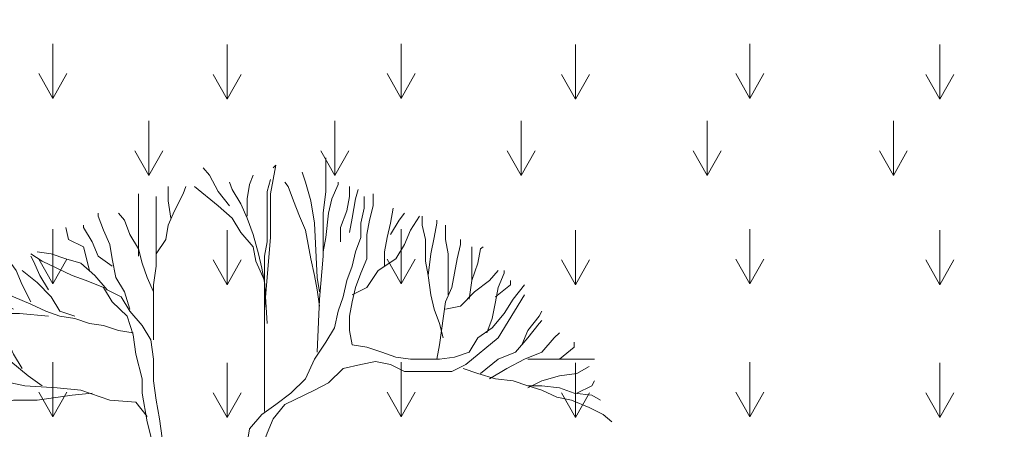
# Model space of a CAD drawing. Units: millimetres. Extents: x 595116 to 630915, y 909473 to 920225.
# Tile 29 of 134: x 629559 to 629622, y 919190 to 919216. Entities that reach past the tile are written whole.
import ezdxf

# ---------------------------------------------------------------- set-up
doc = ezdxf.new("R2010")
doc.units = ezdxf.units.MM
doc.layers.add('Dimension', color=3, linetype='Continuous', lineweight=18)
doc.layers.add('L-PLNT', color=85, linetype='Continuous', lineweight=13)
doc.styles.get("Standard").update_dxf_attribs({"font": 'arial.ttf'})
doc.dimstyles.new('ISO-25', dxfattribs={"dimtxt": 9, "dimasz": 6, "dimexe": 1.25, "dimexo": 0.625, "dimtad": 1, "dimlunit": 4, "dimtxsty": 'Standard', "dimcen": 2.5, "dimadec": 0, "dimazin": 0, "dimtfac": 1, "dimtmove": 0, "dimatfit": 3, "dimfxl": 1, "dimarcsym": 0})

# ---------------------------------------------------------------- blocks, each defined once
blk = doc.blocks.new('A$C143125F4')
for p, q in [((2.5383, 4.8203), (2.5711, 4.9995)), ((2.5711, 4.9995), (2.5547, 4.9816)), ((2.883, 4.8338), (2.883, 5.0443)), ((2.1554, 4.9368), (2.1171, 4.9816)), ((2.2101, 4.8338), (2.1554, 4.9368)), ((2.407, 4.8786), (2.4289, 4.9368)), ((2.7571, 4.892), (2.7353, 4.9547)), ((1.8983, 4.7755), (1.8983, 4.8651)), ((1.9913, 4.8203), (2.0077, 4.8651)), ((2.2101, 4.7442), (2.0624, 4.8651)), ((2.2976, 4.8472), (2.2812, 4.892)), ((2.3906, 4.789), (2.407, 4.8786)), ((2.5164, 4.8338), (2.5383, 4.9099)), ((2.6477, 4.8651), (2.6259, 4.892)), ((2.6806, 4.7755), (2.6477, 4.8651)), ((2.79, 4.7755), (2.7571, 4.892)), ((2.9213, 4.789), (2.9596, 4.8786)), ((2.9596, 4.8786), (2.9596, 4.892)), ((3.0307, 4.8024), (3.0307, 4.8651)), ((1.7123, 4.4306), (1.7123, 4.8203)), ((1.8217, 4.3679), (1.8217, 4.8024)), ((1.9366, 4.7128), (1.9913, 4.8203)), ((2.2812, 4.7442), (2.2101, 4.8338)), ((2.3523, 4.7576), (2.2976, 4.8472)), ((2.5164, 4.5202), (2.5164, 4.8338)), ((2.5383, 4.5471), (2.5383, 4.8203)), ((2.8666, 4.6994), (2.883, 4.8338)), ((3.0143, 4.7128), (3.0307, 4.8024)), ((3.069, 4.789), (3.0854, 4.8472)), ((3.1237, 4.7307), (3.1237, 4.8024)), ((3.1784, 4.7442), (3.1784, 4.8203)), ((1.9147, 4.668), (1.8983, 4.7755)), ((2.2976, 4.668), (2.2101, 4.7442)), ((2.3906, 4.668), (2.3523, 4.7576)), ((2.3906, 4.6814), (2.3906, 4.789)), ((2.7189, 4.6814), (2.6806, 4.7755)), ((2.8119, 4.6367), (2.79, 4.7755)), ((2.8994, 4.6994), (2.9213, 4.789)), ((3.0471, 4.668), (3.069, 4.789)), ((3.1565, 4.6546), (3.1784, 4.7442)), ((1.4606, 4.6814), (1.4606, 4.6994)), ((1.4935, 4.5919), (1.4606, 4.6814)), ((1.6247, 4.6546), (1.5865, 4.6994)), ((1.8983, 4.6232), (1.9366, 4.7128)), ((2.7571, 4.5919), (2.7189, 4.6814)), ((2.8666, 4.4306), (2.8666, 4.6994)), ((2.883, 4.5471), (2.8994, 4.6994)), ((2.976, 4.6098), (3.0143, 4.7128)), ((3.1018, 4.6367), (3.1237, 4.7307)), ((3.2878, 4.6367), (3.3042, 4.7307)), ((3.3425, 4.6546), (3.3753, 4.6994)), ((3.4136, 4.5919), (3.4683, 4.6814)), ((3.4847, 4.6232), (3.4847, 4.6814)), ((1.3676, 4.6098), (1.3676, 4.6232)), ((1.6576, 4.565), (1.6247, 4.6546)), ((1.8819, 4.5336), (1.8983, 4.6232)), ((2.3523, 4.5784), (2.2976, 4.668)), ((2.4289, 4.565), (2.3906, 4.668)), ((2.8283, 4.2962), (2.8119, 4.6367)), ((3.0307, 4.5784), (3.0471, 4.668)), ((3.1018, 4.5471), (3.1018, 4.6367)), ((3.1401, 4.565), (3.1565, 4.6546)), ((3.2659, 4.5471), (3.2878, 4.6367)), ((3.2878, 4.565), (3.3425, 4.6546)), ((3.5066, 4.5336), (3.4847, 4.6232)), ((3.5613, 4.5471), (3.5777, 4.6367)), ((3.5777, 4.6367), (3.5777, 4.6546)), ((3.6324, 4.5336), (3.6324, 4.6232)), ((1.2746, 4.5336), (1.2582, 4.6098)), ((1.4223, 4.5202), (1.3676, 4.6098)), ((1.5317, 4.5023), (1.4935, 4.5919)), ((1.7123, 4.4754), (1.6576, 4.565)), ((2.4289, 4.4888), (2.3523, 4.5784)), ((2.4617, 4.444), (2.4289, 4.565)), ((2.79, 4.4127), (2.7571, 4.5919)), ((2.976, 4.5202), (2.976, 4.6098)), ((3.1401, 4.4127), (3.1401, 4.565)), ((3.3753, 4.5023), (3.4136, 4.5919)), ((1.3676, 4.4888), (1.2746, 4.5336)), ((1.4606, 4.4306), (1.4223, 4.5202)), ((1.5482, 4.4127), (1.5317, 4.5023)), ((1.8217, 4.444), (1.8819, 4.5336)), ((2.5, 4.0991), (2.5383, 4.5471)), ((2.5, 4.4306), (2.5164, 4.5202)), ((2.8666, 4.4575), (2.883, 4.5471)), ((3.069, 4.4575), (3.1018, 4.5471)), ((3.2495, 4.4575), (3.2659, 4.5471)), ((3.3206, 4.4127), (3.3753, 4.5023)), ((3.5066, 4.3992), (3.5066, 4.5336)), ((3.5394, 4.444), (3.5613, 4.5471)), ((3.6488, 4.444), (3.6324, 4.5336)), ((3.7035, 4.4127), (3.7254, 4.5023)), ((3.7254, 4.5023), (3.7254, 4.5336)), ((1.1105, 4.3992), (1.0394, 4.444)), ((1.0777, 4.4575), (1.1652, 4.444)), ((1.1652, 4.444), (1.2582, 4.4127)), ((1.4059, 4.341), (1.3676, 4.4888)), ((1.7342, 4.3858), (1.7123, 4.4754)), ((2.4453, 4.3992), (2.4289, 4.4888)), ((2.4836, 4.3544), (2.4617, 4.444)), ((3.0471, 4.3679), (3.069, 4.4575)), ((3.2495, 4.3679), (3.2495, 4.4575)), ((3.523, 4.3096), (3.5394, 4.444)), ((3.6488, 4.1887), (3.6488, 4.444)), ((3.7965, 4.2783), (3.7965, 4.4888)), ((3.8348, 4.3858), (3.8512, 4.4754)), ((3.8512, 4.4754), (3.8677, 4.4888)), ((0.9464, 4.341), (0.9136, 4.3858)), ((1.0558, 4.3992), (1.0394, 4.4306)), ((1.0941, 4.3096), (1.0558, 4.3992)), ((1.2965, 4.3096), (1.1105, 4.3992)), ((1.2582, 4.4127), (1.3512, 4.3858)), ((1.3512, 4.3858), (1.4387, 4.3096)), ((1.5482, 4.3679), (1.4606, 4.4306)), ((1.57, 4.2962), (1.5482, 4.4127)), ((1.767, 4.2962), (1.7342, 4.3858)), ((2.5, 4.2783), (2.4453, 4.3992)), ((2.5, 3.4584), (2.5, 4.4306)), ((2.8119, 4.3096), (2.79, 4.4127)), ((2.8447, 4.1618), (2.8666, 4.4306)), ((3.1018, 4.3231), (3.1401, 4.4127)), ((3.2112, 4.341), (3.3206, 4.4127)), ((3.523, 4.3096), (3.5066, 4.3992)), ((3.6707, 4.2335), (3.7035, 4.4127)), ((3.7965, 4.2783), (3.8348, 4.3858)), ((0.9847, 4.2514), (0.9464, 4.341)), ((1.0777, 4.2648), (0.9847, 4.341)), ((1.8053, 4.2514), (1.8217, 4.3679)), ((2.5, 4.2648), (2.4836, 4.3544)), ((3.0143, 4.2783), (3.0471, 4.3679)), ((3.069, 4.2335), (3.1018, 4.3231)), ((3.1401, 4.2335), (3.2112, 4.341)), ((3.906, 4.2783), (3.9607, 4.341)), ((3.9607, 4.2335), (3.999, 4.3231)), ((3.999, 4.3231), (3.999, 4.341)), ((0.837, 4.22), (0.8042, 4.2648)), ((1.0394, 4.1439), (0.9847, 4.2514)), ((1.1652, 4.1752), (1.0777, 4.2648)), ((1.1488, 4.22), (1.0941, 4.3096)), ((1.384, 4.2783), (1.2965, 4.3096)), ((1.4935, 4.2335), (1.384, 4.2783)), ((1.4387, 4.3096), (1.5153, 4.22)), ((1.6247, 4.2066), (1.57, 4.2962)), ((1.8053, 4.2066), (1.767, 4.2962)), ((1.8053, 3.9064), (1.8053, 4.2514)), ((2.5164, 4.0095), (2.5, 4.2783)), ((2.8283, 4.22), (2.8119, 4.3096)), ((2.8447, 4.2066), (2.8283, 4.2962)), ((2.9924, 4.1752), (3.0143, 4.2783)), ((3.5394, 4.1887), (3.523, 4.3096)), ((3.7801, 4.1618), (3.7965, 4.2783)), ((3.813, 4.2066), (3.906, 4.2783)), ((3.9442, 4.1752), (4.0372, 4.2514)), ((4.0372, 4.2514), (4.0372, 4.2783)), ((4.1248, 4.2514), (4.0537, 4.1618)), ((0.837, 4.1439), (0.7659, 4.1887)), ((0.93, 4.1752), (0.837, 4.22)), ((1.5482, 4.1439), (1.4935, 4.2335)), ((1.5153, 4.22), (1.6029, 4.1752)), ((1.6576, 4.0991), (1.6247, 4.2066)), ((2.8447, 4.117), (2.8283, 4.22)), ((3.0471, 4.1887), (3.1401, 4.2335)), ((3.0471, 4.1439), (3.069, 4.2335)), ((3.5613, 4.0991), (3.5394, 4.1887)), ((3.6324, 4.1439), (3.6707, 4.2335)), ((3.7254, 4.117), (3.813, 4.2066)), ((3.9442, 4.1439), (3.9607, 4.2335)), ((3.9607, 3.9199), (4.1248, 4.1887)), ((0.6893, 4.117), (0.6729, 4.1304)), ((0.7659, 4.0856), (0.7112, 4.1439)), ((0.93, 4.0991), (0.837, 4.1439)), ((1.0394, 4.1304), (0.93, 4.1752)), ((1.1324, 4.0856), (1.0394, 4.1304)), ((1.2199, 4.0856), (1.1652, 4.1752)), ((1.6412, 4.0543), (1.5482, 4.1439)), ((1.6029, 4.1752), (1.6576, 4.0856)), ((2.8283, 3.8303), (2.8447, 4.1618)), ((2.9596, 4.0856), (2.9924, 4.1752)), ((3.0307, 4.0543), (3.0471, 4.1439)), ((3.5941, 3.8751), (3.6324, 4.1439)), ((3.9224, 4.0408), (3.9442, 4.1439)), ((4.0537, 4.1618), (3.999, 4.0722)), ((0.5635, 4.0274), (0.5252, 4.0722)), ((0.7823, 4.0722), (0.6893, 4.117)), ((0.8206, 3.996), (0.7659, 4.0856)), ((0.9683, 4.0722), (0.7823, 4.0722)), ((1.1488, 4.0543), (0.9683, 4.0722)), ((1.2199, 4.0543), (1.1324, 4.0856)), ((1.3129, 4.0543), (1.2199, 4.0856)), ((1.6576, 4.0856), (1.7342, 3.996)), ((2.5, 3.996), (2.5, 4.0991)), ((2.9377, 3.9826), (2.9596, 4.0856)), ((3.5941, 4.0095), (3.5613, 4.0991)), ((3.6324, 4.0991), (3.7254, 4.117)), ((3.999, 4.0722), (3.9224, 3.9826)), ((4.2178, 4.0543), (4.2342, 4.0856)), ((0.6565, 3.9826), (0.5635, 4.0274)), ((1.3129, 4.0408), (1.2199, 4.0543)), ((1.4059, 4.0095), (1.3129, 4.0408)), ((1.4935, 3.996), (1.4059, 4.0095)), ((1.6795, 3.9378), (1.6412, 4.0543)), ((3.0307, 3.9647), (3.0307, 4.0543)), ((3.616, 3.9199), (3.5941, 4.0095)), ((3.8895, 3.9512), (3.9224, 4.0408)), ((4.1467, 3.9647), (4.2178, 4.0543)), ((4.1467, 3.9199), (4.2178, 4.0095)), ((4.2178, 4.0095), (4.2342, 4.0274)), ((0.6018, 3.9512), (0.5471, 3.996)), ((0.6182, 3.9199), (0.5635, 3.9826)), ((0.6346, 3.8616), (0.6018, 3.9512)), ((0.8206, 3.9647), (0.6565, 3.9826)), ((0.8917, 3.9064), (0.8206, 3.996)), ((1.5865, 3.9647), (1.4935, 3.996)), ((1.6795, 3.9512), (1.5865, 3.9647)), ((1.7342, 3.996), (1.7889, 3.9064)), ((2.883, 3.893), (2.9377, 3.9826)), ((3.0471, 3.8751), (3.0307, 3.9647)), ((3.9224, 3.9826), (3.8348, 3.9199)), ((4.1084, 3.8751), (4.1467, 3.9647)), ((4.3108, 3.9199), (4.3436, 3.9512)), ((0.5088, 3.9199), (0.5088, 3.9378)), ((0.5635, 3.8303), (0.5088, 3.9199)), ((0.7276, 3.8616), (0.6182, 3.9199)), ((0.93, 3.8168), (0.8917, 3.9064)), ((1.6959, 3.8168), (1.6795, 3.9378)), ((1.7889, 3.9064), (1.8053, 3.7855)), ((2.8119, 3.7855), (2.883, 3.893)), ((3.7583, 3.7541), (3.9607, 3.9199)), ((3.8348, 3.9199), (3.7801, 3.8303)), ((4.0701, 3.8303), (4.1467, 3.9199)), ((4.2342, 3.8303), (4.3108, 3.9199)), ((4.4366, 3.8616), (4.4366, 3.893)), ((0.4705, 3.8168), (0.4376, 3.8303)), ((0.6018, 3.7272), (0.5635, 3.8303)), ((0.6893, 3.772), (0.6346, 3.8616)), ((0.9136, 3.772), (0.7276, 3.8616)), ((3.1401, 3.8616), (3.0471, 3.8751)), ((3.2331, 3.8303), (3.1401, 3.8616)), ((3.3206, 3.7989), (3.2331, 3.8303)), ((3.5777, 3.7855), (3.5941, 3.8751)), ((3.7801, 3.8303), (3.6871, 3.7989)), ((3.9607, 3.7855), (4.0701, 3.8303)), ((4.1248, 3.7855), (4.2342, 3.8303)), ((4.3436, 3.7855), (4.4366, 3.8616)), ((0.5635, 3.7407), (0.4705, 3.8168)), ((1.023, 3.6824), (0.9136, 3.772)), ((0.9847, 3.7272), (0.93, 3.8168)), ((1.7342, 3.6645), (1.6959, 3.8168)), ((1.8053, 3.7855), (1.8053, 3.6511)), ((2.7571, 3.6645), (2.8119, 3.7855)), ((3.1018, 3.7541), (3.1948, 3.772)), ((3.1948, 3.772), (3.2878, 3.7541)), ((3.4136, 3.7855), (3.3206, 3.7989)), ((3.5941, 3.7855), (3.4136, 3.7855)), ((3.6871, 3.7989), (3.5941, 3.7855)), ((3.8512, 3.6959), (3.9607, 3.7855)), ((4.0154, 3.7272), (4.1248, 3.7855)), ((4.1467, 3.7855), (4.5624, 3.7855)), ((0.2516, 3.6959), (0.2516, 3.7272)), ((0.3446, 3.6824), (0.2516, 3.6959)), ((0.6565, 3.6959), (0.5635, 3.7407)), ((0.7659, 3.6511), (0.6565, 3.6959)), ((2.8994, 3.6376), (2.9924, 3.7272)), ((2.9924, 3.7272), (3.1018, 3.7541)), ((3.2878, 3.7541), (3.3753, 3.7093)), ((3.3753, 3.7093), (3.6707, 3.7093)), ((3.6707, 3.7093), (3.7583, 3.7541)), ((3.7418, 3.7272), (3.8348, 3.6959)), ((3.8348, 3.6959), (3.9442, 3.6645)), ((3.906, 3.6645), (4.0154, 3.7272)), ((4.3436, 3.6824), (4.453, 3.6959)), ((4.453, 3.6959), (4.5296, 3.7407)), ((0.4923, 3.6645), (0.3446, 3.6824)), ((0.5799, 3.6511), (0.4923, 3.6645)), ((0.7659, 3.6376), (0.5799, 3.6511)), ((0.9136, 3.6376), (0.7659, 3.6376)), ((1.0011, 3.6197), (0.9136, 3.6376)), ((1.1105, 3.6197), (1.023, 3.6824)), ((1.7342, 3.5749), (1.7342, 3.6645)), ((1.8053, 3.6511), (1.8217, 3.5301)), ((2.6641, 3.5749), (2.7571, 3.6645)), ((2.8119, 3.5928), (2.8994, 3.6376)), ((3.9442, 3.6645), (4.0537, 3.6511)), ((4.0537, 3.6511), (4.1467, 3.6197)), ((4.1467, 3.6063), (4.2342, 3.6511)), ((4.2342, 3.6511), (4.3436, 3.6824)), ((4.546, 3.6197), (4.5624, 3.6511)), ((0.1422, 3.6063), (0.1258, 3.6197)), ((0.2352, 3.5749), (0.1422, 3.6063)), ((0.3829, 3.5615), (0.2352, 3.5749)), ((0.3063, 3.5749), (0.3063, 3.5928)), ((0.3993, 3.5301), (0.3063, 3.5749)), ((1.2035, 3.6063), (1.0011, 3.6197)), ((1.3512, 3.5928), (1.2035, 3.6063)), ((1.4223, 3.5749), (1.2965, 3.5615)), ((1.5317, 3.5301), (1.3512, 3.5928)), ((1.767, 3.3957), (1.7342, 3.5749)), ((2.5711, 3.5032), (2.6641, 3.5749)), ((2.6259, 3.5032), (2.8119, 3.5928)), ((4.1467, 3.6197), (4.2342, 3.5928)), ((4.1467, 3.6197), (4.2342, 3.6197)), ((4.2342, 3.6197), (4.3436, 3.6063)), ((4.2342, 3.5928), (4.3272, 3.548)), ((4.3436, 3.6063), (4.4366, 3.5749)), ((4.4366, 3.5749), (4.546, 3.5615)), ((4.453, 3.5749), (4.546, 3.6197)), ((0.5635, 3.5615), (0.3829, 3.5615)), ((0.4923, 3.5032), (0.3993, 3.5301)), ((0.93, 3.5301), (0.8206, 3.5032)), ((1.0777, 3.5301), (0.93, 3.5301)), ((1.2965, 3.5615), (1.0777, 3.5301)), ((1.6959, 3.5167), (1.5317, 3.5301)), ((1.767, 3.4271), (1.6959, 3.5167)), ((1.8217, 3.5301), (1.8436, 3.4136)), ((4.3272, 3.548), (4.4202, 3.5301)), ((4.4202, 3.5301), (4.5296, 3.4853)), ((4.546, 3.5615), (4.6007, 3.5301)), ((0.4376, 3.4584), (0.3446, 3.4405)), ((0.5252, 3.4719), (0.4376, 3.4584)), ((0.5799, 3.4719), (0.4923, 3.5032)), ((0.6182, 3.4719), (0.5252, 3.4719)), ((0.7112, 3.4853), (0.6182, 3.4719)), ((0.8206, 3.5032), (0.7112, 3.4853)), ((2.4836, 3.4405), (2.5711, 3.5032)), ((2.5547, 3.4136), (2.6259, 3.5032)), ((4.5296, 3.4853), (4.6171, 3.4405)), ((0.2516, 3.4271), (0.2188, 3.4271)), ((0.3446, 3.4405), (0.2516, 3.4271)), ((1.7889, 3.3061), (1.767, 3.3957)), ((1.8436, 3.4136), (1.86, 3.2927)), ((2.407, 3.3509), (2.4836, 3.4405)), ((2.5164, 3.3241), (2.5547, 3.4136)), ((4.6171, 3.4405), (4.6718, 3.3957)), ((2.3906, 3.2613), (2.407, 3.3509)), ((1.8053, 3.1897), (1.7889, 3.3061)), ((1.86, 3.2927), (1.8819, 3.2031)), ((2.4836, 3.2345), (2.5164, 3.3241)), ((1.8819, 3.2031), (1.8819, 3.0553)), ((2.3742, 3.1449), (2.3906, 3.2613)), ((2.4836, 3.1449), (2.4836, 3.2345)), ((4.7101, 3.1717), (4.7265, 3.2165)), ((4.7648, 3.1897), (4.7648, 3.2165)), ((1.8217, 3.1001), (1.8053, 3.1897)), ((2.3742, 3.0553), (2.3742, 3.1449)), ((2.5, 3.0553), (2.4836, 3.1449)), ((4.6554, 3.0821), (4.7101, 3.1717)), ((4.7101, 3.1001), (4.7648, 3.1897)), ((1.8436, 2.9925), (1.8217, 3.1001)), ((4.5624, 3.0105), (4.6554, 3.0821)), ((4.6718, 3.0105), (4.7101, 3.1001)), ((4.7648, 3.0373), (4.7812, 3.1001)), ((0.1641, 2.9477), (0.0875, 3.0239)), ((1.8819, 3.0553), (1.9147, 2.9612)), ((2.3359, 2.9612), (2.3742, 3.0553)), ((2.5164, 2.9612), (2.5, 3.0553)), ((4.6718, 2.9477), (4.7648, 3.0373)), ((1.8436, 2.9029), (1.8436, 2.9925)), ((1.9147, 2.9612), (1.9694, 2.8716)), ((2.3359, 2.8716), (2.3359, 2.9612)), ((2.5547, 2.8716), (2.5164, 2.9612)), ((4.5077, 2.9164), (4.5624, 3.0105)), ((4.7265, 2.9164), (4.8195, 2.9791)), ((4.8195, 2.9791), (4.8359, 3.0105)), ((0.1258, 2.9029), (0.0875, 2.9164)), ((0.2188, 2.8716), (0.1258, 2.9029)), ((0.2516, 2.8895), (0.1641, 2.9477)), ((1.86, 2.782), (1.8436, 2.9029)), ((4.453, 2.8133), (4.5077, 2.9164)), ((4.6171, 2.8447), (4.6718, 2.9477)), ((0.1422, 2.7999), (0.0711, 2.8581)), ((0.1094, 2.8268), (0.0711, 2.8581)), ((0.3063, 2.8447), (0.2188, 2.8716)), ((0.3446, 2.7999), (0.2516, 2.8895)), ((1.9694, 2.8716), (2.0077, 2.782)), ((2.3195, 2.782), (2.3359, 2.8716)), ((2.6259, 2.7686), (2.5547, 2.8716)), ((4.5296, 2.7999), (4.639, 2.8447)), ((4.639, 2.8447), (4.7265, 2.8447)), ((4.7265, 2.8447), (4.8031, 2.8895)), ((4.7812, 2.7999), (4.8359, 2.8447)), ((0.1969, 2.782), (0.1094, 2.8268)), ((0.2188, 2.7103), (0.1422, 2.7999)), ((0.3829, 2.6924), (0.1969, 2.782)), ((0.4376, 2.7372), (0.3446, 2.7999)), ((0.7112, 2.7238), (0.6565, 2.782)), ((1.8819, 2.6924), (1.86, 2.782)), ((2.0077, 2.782), (2.0788, 2.6924)), ((2.2648, 2.6924), (2.3195, 2.782)), ((4.3819, 2.679), (4.453, 2.8133)), ((4.4366, 2.7686), (4.5296, 2.7999)), ((4.6937, 2.7238), (4.7812, 2.7999)), ((0.1422, 2.6476), (0.0711, 2.7372)), ((0.2899, 2.6207), (0.2188, 2.7103)), ((0.5252, 2.679), (0.4376, 2.7372)), ((0.8206, 2.6655), (0.7112, 2.7238)), ((2.6806, 2.679), (2.6259, 2.7686)), ((4.6007, 2.6655), (4.6937, 2.7238)), ((4.8359, 2.6924), (4.8359, 2.7103)), ((0.0328, 2.6342), (0.0328, 2.6476)), ((0.2188, 2.5311), (0.1422, 2.6476)), ((0.4705, 2.6924), (0.3829, 2.6924)), ((0.5635, 2.5894), (0.5252, 2.679)), ((0.9136, 2.6028), (0.8206, 2.6655)), ((1.9913, 2.5132), (1.8819, 2.6924)), ((2.0788, 2.6924), (2.1718, 2.6476)), ((2.1718, 2.6476), (2.2648, 2.6924)), ((2.7736, 2.6207), (2.6806, 2.679)), ((3.4683, 2.6207), (3.5613, 2.6655)), ((3.5613, 2.6655), (3.5777, 2.6924)), ((4.3436, 2.5759), (4.3819, 2.679)), ((4.453, 2.6342), (4.5624, 2.6476)), ((4.5624, 2.6476), (4.6554, 2.6655)), ((4.6554, 2.6655), (4.7484, 2.679)), ((4.7484, 2.679), (4.8359, 2.6924)), ((4.8031, 2.558), (4.8578, 2.6476)), ((0.0711, 2.558), (0.0164, 2.5894)), ((0.1258, 2.5894), (0.0328, 2.6342)), ((0.2188, 2.558), (0.1258, 2.5894)), ((0.6346, 2.2444), (0.5635, 2.5894)), ((1.0011, 2.5132), (0.9136, 2.6028)), ((2.8666, 2.6028), (2.7736, 2.6207)), ((2.8666, 2.6028), (3.0854, 2.5759)), ((2.9596, 2.5311), (2.8666, 2.6028)), ((3.2659, 2.5759), (3.3753, 2.5894)), ((3.3753, 2.5894), (3.4683, 2.6207)), ((4.3655, 2.6207), (4.453, 2.6342)), ((0.1641, 2.4863), (0.0711, 2.558)), ((0.3611, 2.3519), (0.2188, 2.5311)), ((0.8917, 2.5446), (0.8753, 2.558)), ((0.9847, 2.4998), (0.8917, 2.5446)), ((3.0471, 2.4684), (2.9596, 2.5311)), ((3.0854, 2.5759), (3.2659, 2.558)), ((3.2659, 2.558), (3.616, 2.558)), ((3.616, 2.558), (3.7965, 2.5446)), ((3.7965, 2.5446), (4.0372, 2.5446)), ((4.0372, 2.5446), (4.1467, 2.558)), ((4.2725, 2.4684), (4.3436, 2.5759)), ((4.6171, 2.4415), (4.8031, 2.558)), ((4.8359, 2.4863), (4.8742, 2.5311)), ((0.0875, 2.455), (0.0328, 2.4998)), ((1.0941, 2.4684), (0.9847, 2.4998)), ((1.2418, 2.455), (1.0941, 2.4684)), ((1.9694, 2.4236), (1.9913, 2.5132)), ((2.8447, 2.4863), (2.7571, 2.4415)), ((2.9377, 2.4415), (2.8447, 2.4863)), ((3.1401, 2.4415), (3.0471, 2.4684)), ((4.1631, 2.4236), (4.2725, 2.4684)), ((4.7484, 2.4415), (4.8359, 2.4863)), ((0.0711, 2.3788), (0, 2.4236)), ((0.1805, 2.4236), (0.0875, 2.455)), ((0.3993, 2.334), (0.1805, 2.4236)), ((0.93, 2.4102), (0.8206, 2.4102)), ((1.023, 2.4236), (0.93, 2.4102)), ((1.1324, 2.4415), (1.023, 2.4236)), ((1.3512, 2.4415), (1.1324, 2.4415)), ((1.3512, 2.4236), (1.2418, 2.455)), ((1.4387, 2.3788), (1.3512, 2.4236)), ((1.8819, 2.3788), (1.9694, 2.4236)), ((2.1007, 2.4236), (2.0077, 2.3967)), ((2.2101, 2.4236), (2.1007, 2.4236)), ((2.3195, 2.4415), (2.2101, 2.4236)), ((2.4289, 2.4236), (2.3195, 2.4415)), ((2.5164, 2.4102), (2.4289, 2.4236)), ((2.5383, 2.3206), (2.5164, 2.4102)), ((2.7571, 2.4415), (2.7189, 2.3519)), ((2.9924, 2.3519), (2.9377, 2.4415)), ((3.2331, 2.3654), (3.1401, 2.4415)), ((4.0537, 2.3654), (4.1631, 2.4236)), ((4.5296, 2.3967), (4.6171, 2.4415)), ((4.5843, 2.4236), (4.9125, 2.4236)), ((4.7812, 2.3788), (4.8578, 2.4102)), ((0.0164, 2.3519), (0.1258, 2.3206)), ((0.1641, 2.3654), (0.0711, 2.3788)), ((0.837, 2.3519), (0.744, 2.3071)), ((0.93, 2.3654), (0.837, 2.3519)), ((1.2965, 2.3654), (0.93, 2.3654)), ((1.4606, 2.3519), (1.2965, 2.3654)), ((1.5482, 2.334), (1.4387, 2.3788)), ((1.8053, 2.2892), (1.8819, 2.3788)), ((2.0077, 2.3967), (1.9694, 2.3071)), ((2.7189, 2.3519), (2.7353, 2.2623)), ((3.069, 2.2623), (2.9924, 2.3519)), ((3.2878, 2.2758), (3.2331, 2.3654)), ((4.0154, 2.2623), (4.0537, 2.3654)), ((4.3436, 2.3071), (4.5296, 2.3967)), ((4.6007, 2.3206), (4.6937, 2.3788)), ((4.6937, 2.3788), (4.7812, 2.3788)), ((0.0547, 2.2623), (0, 2.3071)), ((0.1258, 2.3206), (0.2352, 2.3206)), ((0.2352, 2.3206), (0.3282, 2.3071)), ((0.3282, 2.3071), (0.4158, 2.2758)), ((0.6182, 2.2623), (0.3993, 2.334)), ((1.6412, 2.2444), (1.5482, 2.334)), ((1.7123, 2.231), (1.8053, 2.2892)), ((1.9694, 2.3071), (1.8819, 2.2444)), ((2.5383, 1.8726), (2.5383, 2.3206)), ((4.2561, 2.2758), (4.3436, 2.3071)), ((4.3272, 2.3071), (4.8906, 2.3071)), ((4.8906, 2.3071), (4.9836, 2.2892)), ((4.9836, 2.2892), (4.9836, 2.2758)), ((0.0875, 2.1862), (0.0328, 2.2175)), ((0.1641, 2.2444), (0.0547, 2.2623)), ((0.2516, 2.2175), (0.1641, 2.2444)), ((0.3611, 2.1996), (0.2516, 2.2175)), ((0.4158, 2.2758), (0.6018, 2.2758)), ((0.6018, 2.2758), (0.6893, 2.2444)), ((0.6893, 2.2444), (0.7823, 2.231)), ((0.7823, 2.231), (0.8753, 2.1862)), ((1.6247, 2.1996), (1.7123, 2.231)), ((1.8819, 2.2444), (1.767, 2.1996)), ((2.7353, 2.2623), (2.8119, 2.1727)), ((3.1784, 2.1862), (3.069, 2.2623)), ((3.3753, 2.2175), (3.2878, 2.2758)), ((3.4519, 2.1235), (3.3753, 2.2175)), ((3.4136, 2.1862), (3.5066, 2.231)), ((3.5066, 2.231), (3.616, 2.231)), ((3.616, 2.231), (3.8348, 2.2444)), ((3.8348, 2.2444), (3.999, 2.2623)), ((3.999, 2.2623), (4.1467, 2.2623)), ((4.1467, 2.2623), (4.2561, 2.2758)), ((0.1805, 2.1414), (0.0875, 2.1862)), ((0.6729, 2.1996), (0.3611, 2.1996)), ((0.6182, 2.1862), (0.5252, 2.0966)), ((0.7659, 2.1727), (0.6729, 2.1996)), ((0.8589, 2.1235), (0.7659, 2.1727)), ((0.8753, 2.1862), (0.9136, 2.0966)), ((1.5317, 2.1414), (1.6247, 2.1996)), ((1.767, 2.1996), (1.6959, 2.11)), ((2.8119, 2.1727), (2.8447, 2.0787)), ((3.2495, 2.0966), (3.1784, 2.1862)), ((4.6554, 2.1548), (4.8578, 2.1862)), ((4.8578, 2.1862), (4.8742, 2.1862)), ((0.2735, 2.0518), (0.1805, 2.1414)), ((0.5252, 2.0966), (0.4158, 2.0204)), ((0.8753, 1.9891), (0.8589, 2.1235)), ((0.9136, 2.0966), (0.9464, 2.007)), ((1.4387, 2.0787), (1.5317, 2.1414)), ((1.6959, 2.11), (1.5865, 2.0518)), ((2.6641, 2.1235), (2.6259, 2.0339)), ((2.7571, 2.0787), (2.6641, 2.1235)), ((3.3425, 2.0339), (3.2495, 2.0966)), ((3.5394, 2.0652), (3.4519, 2.1235)), ((4.3436, 2.0787), (4.4749, 2.1235)), ((4.4749, 2.1235), (4.6554, 2.1548)), ((4.5077, 2.1235), (4.6171, 2.1235)), ((4.6171, 2.1235), (4.8031, 2.0966)), ((4.8031, 2.0966), (4.8195, 2.0652)), ((0.1094, 2.0518), (0.0547, 2.0339)), ((0.4541, 2.0518), (0.1094, 2.0518)), ((1.3512, 2.007), (1.4387, 2.0787)), ((1.5865, 2.0518), (1.4935, 2.007)), ((2.6259, 2.0339), (2.6094, 1.9443)), ((2.7736, 1.9891), (2.7571, 2.0787)), ((2.8447, 2.0787), (2.8666, 1.9891)), ((3.3972, 1.9443), (3.3425, 2.0339)), ((3.6324, 2.007), (3.5394, 2.0652)), ((4.1248, 1.9891), (4.2342, 2.0518)), ((4.2342, 2.0518), (4.3436, 2.0787)), ((4.8578, 2.0518), (4.7648, 1.9891)), ((0.2188, 1.9756), (0.0875, 1.9756)), ((0.3282, 1.9622), (0.2188, 1.9756)), ((0.4158, 2.0204), (0.3282, 1.9443)), ((0.8753, 1.8412), (0.8753, 1.9891)), ((0.9464, 2.007), (0.9847, 1.9174)), ((1.2582, 1.9443), (1.3512, 2.007)), ((1.4935, 2.007), (1.384, 1.9174)), ((2.5383, 1.9891), (2.5, 1.8995)), ((2.8283, 1.8995), (2.7736, 1.9891)), ((2.8666, 1.9891), (2.9213, 1.8995)), ((3.7254, 1.9756), (3.6324, 2.007)), ((3.8348, 1.9622), (3.7254, 1.9756)), ((3.9224, 1.9756), (3.8348, 1.9622)), ((4.0154, 1.9443), (3.9224, 1.9756)), ((4.1084, 1.9756), (4.0154, 1.9443)), ((4.2014, 1.9891), (4.1084, 1.9756)), ((4.2014, 1.9756), (4.2014, 1.9891)), ((4.6718, 1.9756), (4.2014, 1.9756)), ((4.7648, 1.9891), (4.6718, 1.9756)), ((4.6937, 1.9622), (4.8031, 1.9756)), ((4.8031, 1.9756), (4.8578, 1.9891)), ((0.3282, 1.9443), (0.2188, 1.886)), ((0.9847, 1.9174), (0.9847, 1.8278)), ((1.1652, 1.886), (1.2582, 1.9443)), ((1.384, 1.9174), (1.2965, 1.8099)), ((2.6094, 1.9443), (2.6094, 1.8547)), ((3.4847, 1.9174), (3.3972, 1.9443)), ((3.4136, 1.9174), (3.5066, 1.886)), ((3.5777, 1.886), (3.4847, 1.9174)), ((4.3108, 1.8726), (4.3983, 1.9174)), ((4.3983, 1.9174), (4.4913, 1.9174)), ((4.4913, 1.9174), (4.5843, 1.9443)), ((4.5843, 1.9443), (4.6937, 1.9622)), ((4.7265, 1.9308), (4.6171, 1.886)), ((4.8195, 1.9622), (4.7265, 1.9308)), ((0.2188, 1.886), (0.1258, 1.8278)), ((0.2735, 1.886), (0.1805, 1.7964)), ((1.0777, 1.8278), (1.1652, 1.886)), ((2.5, 1.8995), (2.2976, 1.7516)), ((2.5164, 1.783), (2.5383, 1.8726)), ((2.6094, 1.8547), (2.593, 1.7651)), ((2.8994, 1.8099), (2.8283, 1.8995)), ((2.9213, 1.8995), (2.9924, 1.8099)), ((3.5066, 1.886), (3.5777, 1.7964)), ((3.6707, 1.8726), (3.5777, 1.886)), ((3.7583, 1.8547), (3.6707, 1.8726)), ((3.8512, 1.8412), (3.7583, 1.8547)), ((4.0372, 1.8547), (3.9442, 1.8412)), ((4.1248, 1.8547), (4.0372, 1.8547)), ((4.5296, 1.8547), (4.1248, 1.8547)), ((4.2178, 1.8547), (4.3108, 1.8726)), ((4.6171, 1.886), (4.5296, 1.8547)), ((0.1258, 1.8278), (0.0875, 1.7964)), ((0.1805, 1.7964), (0.1422, 1.7382)), ((0.8206, 1.7516), (0.8753, 1.8412)), ((0.9847, 1.8278), (1.0777, 1.8278)), ((1.2965, 1.8099), (1.1488, 1.7516)), ((2.5383, 1.7964), (2.4617, 1.6934)), ((2.976, 1.7203), (2.8994, 1.8099)), ((2.9924, 1.8099), (3.0854, 1.7382)), ((3.5777, 1.7964), (3.6871, 1.7516)), ((3.9442, 1.8412), (3.8512, 1.8412)), ((4.3272, 1.8412), (4.453, 1.7964)), ((4.453, 1.7964), (4.546, 1.7516)), ((4.6171, 1.8099), (4.7101, 1.7964)), ((4.7101, 1.7964), (4.7812, 1.7651)), ((0.3282, 1.7516), (0.2188, 1.7203)), ((0.4376, 1.7651), (0.3282, 1.7516)), ((0.837, 1.7651), (0.4376, 1.7651)), ((0.6182, 1.7651), (0.4541, 1.7203)), ((0.7276, 1.662), (0.8206, 1.7516)), ((1.1488, 1.7516), (0.9683, 1.6934)), ((1.1488, 1.7516), (1.0777, 1.662)), ((2.2976, 1.7516), (2.1882, 1.662)), ((2.5164, 1.6934), (2.5164, 1.783)), ((2.593, 1.7651), (2.593, 1.3932)), ((3.0854, 1.7382), (3.1948, 1.559)), ((3.6871, 1.7516), (3.7801, 1.7203)), ((4.546, 1.7516), (4.639, 1.6755)), ((0.2188, 1.7203), (0.1422, 1.6755)), ((0.4541, 1.7203), (0.3063, 1.6486)), ((0.3993, 1.6755), (0.3282, 1.5859)), ((0.9683, 1.6934), (0.7823, 1.6172)), ((2.4617, 1.6934), (2.3906, 1.5724)), ((2.5, 1.559), (2.5164, 1.6934)), ((3.069, 1.6486), (2.976, 1.7203)), ((3.7801, 1.7203), (3.999, 1.662)), ((3.8677, 1.6934), (3.9442, 1.5724)), ((4.639, 1.6755), (4.7101, 1.6307)), ((0.1969, 1.6038), (0.1258, 1.5724)), ((0.3063, 1.6486), (0.1969, 1.6038)), ((0.5252, 1.559), (0.6346, 1.6038)), ((0.7823, 1.6172), (0.6018, 1.559)), ((0.6346, 1.6038), (0.7276, 1.662)), ((1.0777, 1.662), (1.0011, 1.5724)), ((1.023, 1.6172), (1.023, 1.5142)), ((2.1007, 1.6172), (2.0241, 1.5276)), ((2.1882, 1.662), (2.1007, 1.6172)), ((3.1018, 1.5411), (3.069, 1.6486)), ((3.999, 1.662), (4.1795, 1.5859)), ((4.0701, 1.6307), (4.1631, 1.6172)), ((4.1631, 1.6172), (4.5296, 1.6172)), ((4.5296, 1.6172), (4.6171, 1.6038)), ((4.6171, 1.6038), (4.7101, 1.6172)), ((0.3282, 1.5859), (0.3063, 1.4963)), ((0.3446, 1.5142), (0.4376, 1.5411)), ((0.4376, 1.5411), (0.5252, 1.559)), ((0.6018, 1.559), (0.5088, 1.4828)), ((1.0011, 1.5724), (0.9136, 1.4515)), ((2.3906, 1.5724), (2.3359, 1.438)), ((2.4617, 1.4694), (2.5, 1.559)), ((3.1237, 1.4515), (3.1018, 1.5411)), ((3.1948, 1.559), (3.2112, 1.4694)), ((3.9442, 1.5724), (4.0372, 1.4694)), ((4.1795, 1.5859), (4.2725, 1.559)), ((4.2178, 1.5724), (4.3108, 1.5276)), ((4.2725, 1.559), (4.4202, 1.5411)), ((4.4202, 1.5411), (4.5077, 1.4963)), ((0.2735, 1.4246), (0.3446, 1.5142)), ((0.3063, 1.4963), (0.2735, 1.438)), ((0.5088, 1.4828), (0.3993, 1.4067)), ((1.023, 1.5142), (1.0011, 1.3932)), ((2.0241, 1.5276), (1.9366, 1.4515)), ((3.999, 1.5276), (4.1084, 1.4515)), ((4.3108, 1.5276), (4.3983, 1.4828)), ((4.3983, 1.4828), (4.4749, 1.3798)), ((4.4749, 1.5142), (4.6718, 1.5142)), ((4.5077, 1.4963), (4.5843, 1.4067)), ((0.9136, 1.4515), (0.7276, 1.3619)), ((0.9136, 1.438), (0.8753, 1.3036)), ((1.8436, 1.4246), (1.7506, 1.3798)), ((1.9366, 1.4515), (1.8436, 1.4246)), ((1.9366, 1.4694), (1.9147, 1.3798)), ((2.3359, 1.438), (2.2429, 1.2857)), ((2.4453, 1.3798), (2.4617, 1.4694)), ((3.1565, 1.3619), (3.1237, 1.4515)), ((3.2112, 1.4694), (3.2331, 1.3798)), ((4.0372, 1.4694), (4.1248, 1.3932)), ((4.1084, 1.4515), (4.2178, 1.4067)), ((0.2899, 1.3798), (0.2516, 1.3619)), ((0.3993, 1.4067), (0.2899, 1.3798)), ((0.7276, 1.3619), (0.6182, 1.3171)), ((0.8042, 1.4067), (0.7659, 1.2857)), ((1.0011, 1.3932), (1.0011, 1.2723)), ((1.6576, 1.3619), (1.4387, 1.2723)), ((1.7506, 1.3798), (1.6576, 1.3619)), ((1.8436, 1.4067), (1.6959, 1.335)), ((1.9147, 1.3798), (1.8053, 1.2857)), ((2.2429, 1.3798), (2.1007, 1.3171)), ((2.3906, 1.2857), (2.4453, 1.3798)), ((2.593, 1.3932), (2.4836, 1.214)), ((3.2331, 1.1827), (3.1565, 1.3619)), ((3.2331, 1.3798), (3.2495, 1.2409)), ((4.1084, 1.3932), (4.2014, 1.3619)), ((4.1248, 1.3932), (4.1795, 1.2857)), ((4.2014, 1.3619), (4.2889, 1.335)), ((4.2178, 1.4067), (4.3108, 1.3932)), ((4.3108, 1.3932), (4.3983, 1.3619)), ((4.3983, 1.3619), (4.4913, 1.3171)), ((4.4749, 1.3798), (4.546, 1.2857)), ((0.3446, 1.335), (0.2516, 1.3484)), ((0.6729, 1.335), (0.3446, 1.335)), ((0.6182, 1.3171), (0.5252, 1.2588)), ((0.8753, 1.3036), (0.8589, 1.1961)), ((1.6959, 1.335), (1.4935, 1.1692)), ((1.8983, 1.3036), (1.7506, 1.2857)), ((2.1007, 1.3171), (1.8983, 1.3036)), ((2.1335, 1.335), (2.0624, 1.2409)), ((4.2889, 1.335), (4.3819, 1.2723)), ((4.4913, 1.3171), (4.546, 1.2857)), ((0.5252, 1.2588), (0.4376, 1.2275)), ((0.5471, 1.2723), (0.5088, 1.1827)), ((0.7659, 1.2857), (0.6729, 1.2275)), ((1.0011, 1.2723), (0.9847, 1.1379)), ((1.3293, 1.2409), (1.2418, 1.1827)), ((1.4387, 1.2723), (1.3293, 1.2409)), ((1.5865, 1.2723), (1.4935, 1.1692)), ((1.7506, 1.2857), (1.5865, 1.2723)), ((1.8053, 1.2857), (1.6959, 1.1692)), ((2.0624, 1.2409), (1.953, 1.1513)), ((2.2429, 1.2857), (2.1718, 1.1827)), ((2.3906, 1.1961), (2.3906, 1.2857)), ((3.2495, 1.2409), (3.2659, 1.1513)), ((4.1795, 1.2857), (4.2725, 1.2275)), ((4.2014, 1.2409), (4.2178, 1.1244)), ((4.3819, 1.2723), (4.4749, 1.2275)), ((0.4376, 1.2275), (0.3993, 1.214)), ((0.5088, 1.1827), (0.4923, 1.0931)), ((0.6729, 1.2275), (0.5635, 1.1513)), ((0.8589, 1.1961), (0.7823, 1.1065)), ((1.0011, 1.2275), (0.9136, 1.1513)), ((1.2418, 1.1827), (1.1488, 1.1244)), ((2.1718, 1.1827), (2.0624, 1.0483)), ((2.3906, 1.2275), (2.2265, 0.9587)), ((2.3742, 1.1065), (2.3906, 1.1961)), ((2.4836, 1.214), (2.4453, 1.1244)), ((3.2659, 1.0035), (3.2331, 1.1827)), ((4.2725, 1.2275), (4.3436, 1.1379)), ((4.4749, 1.2275), (4.5077, 1.214)), ((0.5635, 1.1513), (0.5088, 1.1065)), ((0.8042, 1.1379), (0.7112, 1.0931)), ((0.9136, 1.1513), (0.8206, 1.0796)), ((0.9847, 1.1379), (0.9683, 1.0169)), ((1.1488, 1.1244), (1.0558, 1.0483)), ((1.1871, 1.1244), (1.1652, 1.0169)), ((1.4935, 1.1692), (1.384, 1.1065)), ((1.4935, 1.1692), (1.4223, 1.0483)), ((1.57, 1.1244), (1.477, 1.0348)), ((1.6959, 1.1692), (1.57, 1.1244)), ((1.953, 1.1513), (1.86, 1.0617)), ((2.4453, 1.1244), (2.407, 1.0931)), ((3.2659, 1.1513), (3.3042, 1.0617)), ((4.2178, 1.1244), (4.2342, 1.0348)), ((4.3436, 1.1379), (4.3983, 1.0483)), ((0.5252, 1.0617), (0.4541, 1.0483)), ((0.4923, 1.0931), (0.4705, 1.0931)), ((0.6182, 1.0931), (0.5252, 1.0617)), ((0.7112, 1.0931), (0.6182, 1.0931)), ((0.7823, 1.1065), (0.6893, 1.0169)), ((0.8206, 1.0796), (0.7659, 0.99)), ((1.0558, 1.0483), (0.9136, 0.8691)), ((1.2965, 1.0483), (1.2199, 0.9452)), ((1.384, 1.1065), (1.2965, 1.0483)), ((1.4223, 1.0483), (1.3512, 0.9452)), ((1.6795, 1.0483), (1.477, 0.9721)), ((1.86, 1.0617), (1.6795, 1.0483)), ((2.0624, 1.0483), (2.0077, 0.9273)), ((2.3742, 1.0169), (2.3742, 1.1065)), ((2.407, 1.0931), (2.3906, 1.0035)), ((2.4289, 1.0796), (2.4453, 0.9587)), ((3.2495, 1.0796), (3.2495, 0.5869)), ((3.3042, 1.1065), (3.3425, 1.0169)), ((3.3042, 1.0617), (3.3206, 0.9587)), ((4.2178, 1.0796), (4.3108, 1.0796)), ((4.3108, 1.0796), (4.3819, 1.0348)), ((4.3983, 1.0483), (4.4202, 1.0348)), ((0.6893, 1.0169), (0.6018, 0.9721)), ((0.7659, 0.99), (0.6893, 0.9005)), ((0.8042, 1.0348), (0.7823, 0.9452)), ((0.9683, 0.99), (0.8589, 0.9273)), ((0.9683, 1.0169), (0.9683, 0.9273)), ((1.1652, 1.0169), (1.1324, 0.9273)), ((1.384, 0.99), (1.2965, 0.9452)), ((1.477, 1.0348), (1.384, 0.99)), ((2.3523, 0.9273), (2.3742, 1.0169)), ((2.3906, 1.0035), (2.3906, 0.6765)), ((3.3042, 0.9139), (3.2659, 1.0035)), ((3.3425, 1.0169), (3.43, 0.9721)), ((4.2342, 1.0348), (4.2725, 0.9452)), ((0.6018, 0.9721), (0.5635, 0.9273)), ((0.7823, 0.9452), (0.7276, 0.8557)), ((0.8589, 0.9273), (0.7823, 0.8377)), ((0.8753, 0.9452), (0.8589, 0.8557)), ((0.9683, 0.9273), (0.93, 0.8109)), ((1.1324, 0.9273), (1.0941, 0.8243)), ((1.2199, 0.9452), (1.1324, 0.9005)), ((1.3293, 0.9587), (1.1871, 0.9005)), ((1.2965, 0.9452), (1.2199, 0.8243)), ((1.3512, 0.9452), (1.2582, 0.8557)), ((1.477, 0.9721), (1.3293, 0.9587)), ((1.9913, 0.9273), (1.7889, 0.8825)), ((2.0077, 0.9273), (1.953, 0.8243)), ((2.2265, 0.9587), (2.1554, 0.8377)), ((2.3523, 0.8377), (2.3523, 0.9273)), ((2.4453, 0.9587), (2.4617, 0.8691)), ((3.3206, 0.9587), (3.3753, 0.8691)), ((3.43, 0.9721), (3.523, 0.9587)), ((3.523, 0.9587), (3.6324, 0.9452)), ((3.6324, 0.9452), (3.7418, 0.9452)), ((3.6871, 0.9452), (3.7418, 0.8557)), ((3.7418, 0.9452), (3.8512, 0.9273)), ((3.8512, 0.9273), (3.9607, 0.9005)), ((4.2725, 0.9452), (4.2889, 0.9005)), ((0.6893, 0.9005), (0.6346, 0.8557)), ((0.9136, 0.8691), (0.8753, 0.7795)), ((1.1324, 0.9005), (0.9464, 0.7481)), ((1.1871, 0.9005), (1.0011, 0.8377)), ((1.7889, 0.8825), (1.6029, 0.8377)), ((2.4617, 0.8691), (2.5, 0.7347)), ((3.3206, 0.8243), (3.3042, 0.9139)), ((3.3753, 0.8691), (3.43, 0.7481)), ((3.9607, 0.9005), (4.0537, 0.8691)), ((4.0537, 0.8691), (4.1467, 0.8557)), ((0.7276, 0.8557), (0.7112, 0.7795)), ((0.7823, 0.8377), (0.744, 0.7795)), ((1.0011, 0.8377), (0.7823, 0.7481)), ((0.8589, 0.8557), (0.837, 0.7661)), ((0.93, 0.8109), (0.9136, 0.7213)), ((1.0941, 0.8243), (1.0011, 0.7347)), ((1.2199, 0.8243), (1.1324, 0.7347)), ((1.2582, 0.8557), (1.2035, 0.7661)), ((1.3676, 0.8243), (1.2582, 0.7929)), ((1.4606, 0.8243), (1.3676, 0.8243)), ((1.4223, 0.8243), (1.384, 0.5555)), ((1.6029, 0.8377), (1.4606, 0.8243)), ((1.6795, 0.8557), (1.6029, 0.7661)), ((1.953, 0.8243), (1.86, 0.7033)), ((2.1554, 0.8377), (2.1171, 0.7481)), ((2.3523, 0.8243), (2.2976, 0.7347)), ((2.3359, 0.7481), (2.3523, 0.8377)), ((3.3589, 0.7347), (3.3206, 0.8243)), ((3.7418, 0.8557), (3.8512, 0.8109)), ((3.8512, 0.8109), (3.9442, 0.7661)), ((4.1467, 0.8557), (4.2014, 0.8243)), ((0.7823, 0.7481), (0.6893, 0.6899)), ((0.837, 0.7661), (0.8042, 0.6765)), ((0.8753, 0.7795), (0.8589, 0.7481)), ((1.023, 0.7795), (0.93, 0.7033)), ((0.9464, 0.7481), (0.9464, 0.7347)), ((1.1105, 0.7929), (1.023, 0.7795)), ((1.2582, 0.7929), (1.1105, 0.7929)), ((1.2035, 0.7661), (1.1652, 0.6899)), ((1.2746, 0.7929), (1.2035, 0.7033)), ((1.6029, 0.7661), (1.5482, 0.6765)), ((2.1171, 0.7481), (2.0241, 0.6137)), ((2.3359, 0.3897), (2.3359, 0.7481)), ((3.43, 0.7481), (3.5394, 0.6585)), ((3.906, 0.7929), (3.999, 0.7795)), ((3.9442, 0.7661), (4.0154, 0.6765)), ((3.999, 0.7795), (4.092, 0.7929)), ((4.092, 0.7929), (4.1795, 0.7795)), ((0.6893, 0.6899), (0.6893, 0.6765)), ((0.93, 0.7033), (0.8753, 0.6451)), ((0.9136, 0.7213), (0.8917, 0.6317)), ((1.0011, 0.7347), (0.9464, 0.6451)), ((1.1324, 0.7347), (1.0941, 0.6899)), ((1.2035, 0.7033), (1.0941, 0.6317)), ((1.86, 0.7033), (1.767, 0.6137)), ((2.2976, 0.7347), (2.2812, 0.6451)), ((2.5, 0.7347), (2.5383, 0.6451)), ((3.4519, 0.6451), (3.3589, 0.7347)), ((3.3972, 0.7033), (3.4136, 0.6137)), ((0.8042, 0.6765), (0.8042, 0.6585)), ((0.8917, 0.6317), (0.8753, 0.6317)), ((1.0941, 0.6317), (0.9847, 0.5421)), ((1.5482, 0.6765), (1.5482, 0.6451)), ((1.8217, 0.6585), (1.7506, 0.5421)), ((2.0241, 0.6317), (1.9366, 0.5421)), ((2.2812, 0.6451), (2.2648, 0.5107)), ((2.3906, 0.6765), (2.3742, 0.5689)), ((2.5164, 0.6585), (2.6094, 0.5421)), ((2.5383, 0.6451), (2.6477, 0.4659)), ((3.5394, 0.5689), (3.4519, 0.6451)), ((3.5394, 0.6765), (3.7801, 0.6451)), ((3.5394, 0.6585), (3.6488, 0.5869)), ((3.7801, 0.6451), (3.9442, 0.6317)), ((3.9442, 0.6317), (4.0372, 0.6451)), ((4.0154, 0.6765), (4.0537, 0.6585)), ((1.767, 0.6137), (1.6795, 0.5241)), ((2.0241, 0.6137), (1.953, 0.5241)), ((2.3742, 0.5689), (2.3742, 0.4525)), ((3.2495, 0.5869), (3.3042, 0.4973)), ((3.2495, 0.5869), (3.2659, 0.4973)), ((3.4136, 0.6137), (3.5777, 0.3449)), ((3.7254, 0.4525), (3.5394, 0.5689)), ((3.5777, 0.5555), (3.6488, 0.4659)), ((3.6488, 0.5869), (3.7418, 0.5241)), ((1.6795, 0.5241), (1.6247, 0.3897)), ((1.7506, 0.5421), (1.6959, 0.4032)), ((1.953, 0.5241), (1.7889, 0.2554)), ((1.9366, 0.5421), (1.8217, 0.4525)), ((2.2648, 0.5107), (2.2265, 0.3763)), ((2.407, 0.5107), (2.407, 0.4211)), ((2.6094, 0.5421), (2.7571, 0.4659)), ((3.2659, 0.4973), (3.2878, 0.4032)), ((3.3042, 0.4973), (3.3753, 0.4032)), ((3.4847, 0.4973), (3.4847, 0.3763)), ((3.7418, 0.5241), (3.8348, 0.4793)), ((1.0777, 0.4211), (1.0558, 0.4345)), ((1.6795, 0.4793), (1.4935, 0.4032)), ((1.8217, 0.4525), (1.767, 0.3584)), ((1.953, 0.4793), (1.8983, 0.3897)), ((2.3523, 0.3584), (2.3742, 0.4793)), ((2.3742, 0.4793), (2.3523, 0.3763)), ((2.3742, 0.4525), (2.3523, 0.3584)), ((2.6477, 0.4659), (2.7189, 0.3763)), ((2.7571, 0.4659), (2.8994, 0.4211)), ((3.3425, 0.4525), (3.3753, 0.3584)), ((3.6488, 0.4659), (3.7254, 0.3763)), ((3.813, 0.4211), (3.7254, 0.4525)), ((3.8348, 0.4793), (3.8677, 0.4659)), ((1.1871, 0.4032), (1.0777, 0.4211)), ((1.2746, 0.4032), (1.1871, 0.4032)), ((1.3129, 0.3897), (1.2418, 0.3584)), ((1.384, 0.3897), (1.2746, 0.4032)), ((1.4935, 0.4032), (1.3129, 0.3897)), ((1.4935, 0.4032), (1.4606, 0.3136)), ((1.6247, 0.3897), (1.5482, 0.3002)), ((1.6959, 0.4032), (1.6412, 0.3136)), ((1.8983, 0.3897), (1.86, 0.2554)), ((1.9147, 0.3763), (1.9147, 0.2867)), ((2.2265, 0.3763), (2.2101, 0.2419)), ((2.3195, 0.3002), (2.3359, 0.3897)), ((2.3523, 0.3763), (2.3523, 0.3449)), ((2.407, 0.4211), (2.4453, 0.3315)), ((2.7189, 0.3763), (2.7571, 0.2867)), ((2.8447, 0.4211), (2.8666, 0.3315)), ((2.8994, 0.4211), (3.0143, 0.3763)), ((3.0143, 0.3763), (3.1018, 0.3584)), ((3.2878, 0.4032), (3.3206, 0.224)), ((3.3753, 0.4032), (3.4519, 0.3136)), ((3.4847, 0.3763), (3.5066, 0.2867)), ((3.7254, 0.3763), (3.7254, 0.3584)), ((1.4606, 0.3136), (1.4059, 0.2867)), ((1.6412, 0.3136), (1.5865, 0.1792)), ((1.767, 0.3584), (1.6959, 0.2688)), ((2.2265, 0.3315), (2.1718, 0.2419)), ((2.3523, 0.3449), (2.3359, 0.2554)), ((2.4453, 0.3315), (2.4617, 0.2419)), ((2.7189, 0.3136), (2.7353, 0.2106)), ((2.8666, 0.3315), (2.9596, 0.2688)), ((3.1018, 0.3584), (3.1948, 0.2867)), ((3.3753, 0.3584), (3.4136, 0.2688)), ((3.5777, 0.3449), (3.5941, 0.3136)), ((1.5482, 0.3002), (1.5317, 0.2688)), ((1.6959, 0.2688), (1.6576, 0.224)), ((1.7889, 0.2554), (1.7123, 0.1971)), ((1.86, 0.2554), (1.86, 0.1658)), ((1.9147, 0.2867), (1.9366, 0.1971)), ((2.2101, 0.2554), (2.1882, 0.1344)), ((2.3195, 0.2106), (2.3195, 0.3002)), ((2.3359, 0.2554), (2.3359, 0)), ((2.4836, 0.2688), (2.5711, 0.2106)), ((2.7571, 0.2867), (2.8119, 0.1971)), ((2.9596, 0.2688), (3.0471, 0.1792)), ((3.1948, 0.2867), (3.2659, 0.224)), ((3.4136, 0.2688), (3.43, 0.2419)), ((1.9366, 0.1971), (1.9366, 0.0896)), ((2.1718, 0.2419), (2.1007, 0.1523)), ((2.2101, 0.2419), (2.1335, 0.1523)), ((2.2976, 0.121), (2.3195, 0.2106)), ((2.4617, 0.2419), (2.5, 0.1523)), ((2.5711, 0.2106), (2.6477, 0.121)), ((2.7353, 0.2106), (2.7736, 0.121)), ((2.79, 0.2419), (2.8994, 0.1971)), ((2.8119, 0.1971), (2.8994, 0.1075)), ((2.8994, 0.1971), (2.976, 0.1075)), ((3.3206, 0.224), (3.3425, 0.1971)), ((1.5865, 0.1792), (1.57, 0.121)), ((1.86, 0.1658), (1.8217, 0.121)), ((2.1007, 0.1523), (2.0241, 0.121)), ((2.1335, 0.1523), (2.1007, 0.0762)), ((2.1882, 0.1344), (2.1718, 0.0896)), ((2.5, 0.1658), (2.4836, 0.0762)), ((2.5, 0.1523), (2.5164, 0.0627)), ((3.0471, 0.1792), (3.0854, 0.1658)), ((2.2976, 0.0179), (2.2976, 0.121)), ((2.4836, 0.0762), (2.4617, 0.0448)), ((2.5164, 0.0627), (2.5164, 0.0448)), ((2.6477, 0.121), (2.7024, 0.0448)), ((2.7736, 0.121), (2.8119, 0.0627)), ((2.8994, 0.1075), (2.976, 0.0314)), ((2.976, 0.1075), (3.0143, 0.0762))]:
    blk.add_line(p, q)
blk = doc.blocks.new('LAWN-GRASS-TUFT')
blk.add_line((0.892, 3.485), (0.892, 0))
blk.add_lwpolyline([(0, 1.577), (0.892, 0), (1.785, 1.577)])
blk = doc.blocks.new('*D216')
at = {"layer": 'Defpoints', "color": 0, "transparency": 16777216}
for p in [(629505.041, 919411.828), (629743.541, 919411.928), (629743.541, 918832.378)]:
    blk.add_point(p, dxfattribs=at)
at = {"layer": 'Dimension', "color": 0, "lineweight": -2, "transparency": 16777216}
for p, q in [((629505.041, 919411.203), (629505.041, 918831.128)), ((629743.541, 919411.303), (629743.541, 918831.128)), ((629511.041, 918832.378), (629737.541, 918832.378))]:
    blk.add_line(p, q, dxfattribs=at)
at = {"layer": 'Dimension', "color": 0, "transparency": 16777216}
for points in [[(629511.041, 918833.378), (629511.041, 918831.378), (629505.041, 918832.378)], [(629737.541, 918833.378), (629737.541, 918831.378), (629743.541, 918832.378)]]:
    blk.add_solid(points, dxfattribs=at)
at = {"layer": 'Dimension', "color": 0, "transparency": 16777216, "insert": (629624.291, 918837.656), "char_height": 9, "attachment_point": 5}
blk.add_mtext('19\'-10 1/2"', dxfattribs=at)

msp = doc.modelspace()

# ---------------------------------------------------------------- block references
at = {"layer": 'L-PLNT'}
for p in [(629560.321, 919211.374), (629571.434, 919211.325), (629582.548, 919211.374), (629593.662, 919211.325), (629604.776, 919211.374), (629616.912, 919211.325), (629566.446, 919206.447), (629578.319, 919206.447), (629590.192, 919206.447), (629602.065, 919206.447), (629613.938, 919206.447), (629560.321, 919199.536), (629571.434, 919199.487), (629582.548, 919199.536), (629593.662, 919199.487), (629604.776, 919199.536), (629616.912, 919199.487), (629560.321, 919191.067), (629571.434, 919191.017), (629582.548, 919191.067), (629593.662, 919191.017), (629604.776, 919191.067), (629616.912, 919191.017)]:
    msp.add_blockref('LAWN-GRASS-TUFT', p, dxfattribs=at)
at = {"layer": 'L-PLNT', "xscale": 10.20167662382051, "yscale": 10.20167662382051, "zscale": 10.20167662382051}
msp.add_blockref('A$C143125F4', (629549.214, 919156.111), dxfattribs=at)

# ---------------------------------------------------------------- dimensions: what is measured, and where the dimension line sits
at = {"layer": 'Dimension'}
dim = msp.add_linear_dim(base=(629743.541, 918832.378), p1=(629505.041, 919411.828), p2=(629743.541, 919411.928), dimstyle='ISO-25', override={"dimdec": 1, "dimlfac": 1, "dimrnd": 0, "dimzin": 1, "dimdsep": 46, "dimlunit": 4, "dimfrac": 2}, dxfattribs=at)
dim.commit()
dim.dimension.update_dxf_attribs({"geometry": '*D216', "text_midpoint": (629624.291, 918837.656)})

doc.saveas('drawing.dxf')
